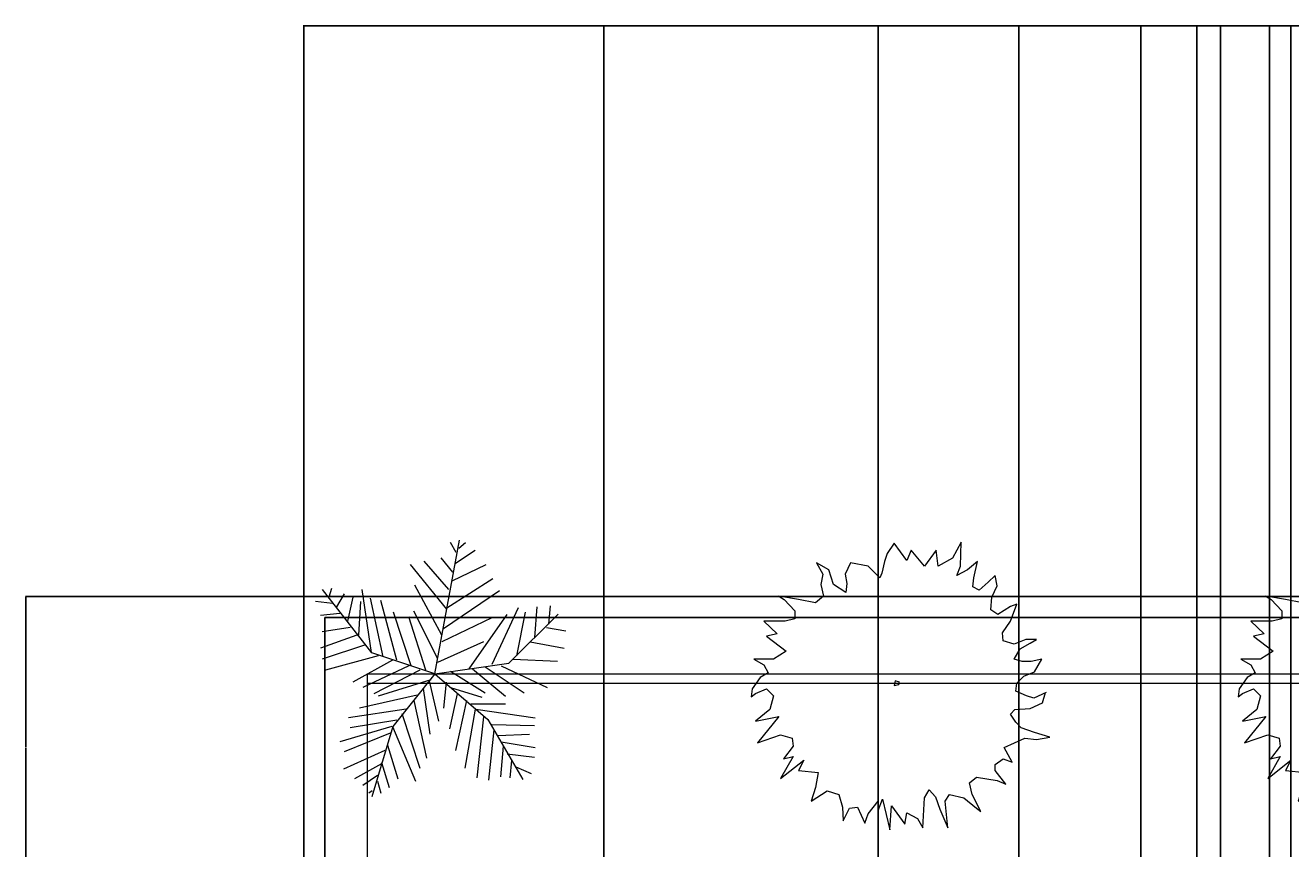
# Model space of a CAD drawing. Units: inches. Extents: x -4843 to -3402, y -164 to 3629.
# Tile 18 of 22: x -4843 to -4303, y 1042 to 1393. Entities that reach past the tile are written whole.
import ezdxf

# ---------------------------------------------------------------- set-up
doc = ezdxf.new("R2010")
doc.units = ezdxf.units.IN
for name, color, linetype, lineweight in [('A-ANNO-DIMS', 2, 'Continuous', 18), ('C-PROP', 7, 'Continuous', 25), ('L-PLNT-EDGE', 7, 'Continuous', 18), ('PLANTS', 3, 'Continuous', 13)]:
    doc.layers.add(name, color=color, linetype=linetype, lineweight=lineweight)
doc.styles.get("Standard").update_dxf_attribs({"font": 'arial.ttf'})
doc.dimstyles.get("Standard").update_dxf_attribs({"dimtxt": 0.18, "dimasz": 0.18, "dimexe": 0.18, "dimexo": 0.0625, "dimgap": 0.09, "dimtad": 0, "dimtih": 1, "dimtoh": 1, "dimdec": 4, "dimzin": 0, "dimdsep": 46, "dimtxsty": 'Standard', "dimcen": 0.09, "dimadec": 0, "dimazin": 0, "dimtfac": 1, "dimtdec": 4, "dimtofl": 0, "dimtmove": 0, "dimatfit": 3, "dimfxl": 1, "dimtolj": 1, "dimtzin": 0, "dimarcsym": 0})

# ---------------------------------------------------------------- blocks, each defined once
blk = doc.blocks.new('*U33')
for p, q in [((-258.7244, 1362.456), (-332.3336, 1421.4348)), ((0, 0), (-266.7, 1447.8)), ((-231.1146, 1315.2628), (-166.7002, 1421.4348)), ((-221.9198, 1197.3052), (-433.5526, 1338.8594)), ((-194.31, 1102.9442), (-65.4812, 1256.284)), ((-185.1152, 1008.5578), (-553.1612, 1185.4942)), ((-148.3106, 914.1968), (118.5418, 1220.9018)), ((-129.8956, 701.8528), (265.7602, 1185.4942)), ((-129.8956, 713.6638), (-626.7704, 1032.1544)), ((-74.7014, 418.7444), (219.7608, 961.39)), ((-93.091, 489.5342), (-700.3796, 902.3858)), ((685.8, 228.6), (1219.2, 914.4)), ((689.0258, 230.0224), (790.2448, 914.1968)), ((891.4384, 831.6214), (946.658, 572.1096)), ((983.4626, 867.0036), (1066.2666, 725.4494)), ((1121.4862, 925.9824), (1149.0706, 831.6214)), ((-1234.059, 536.7274), (-1252.4486, 737.2604)), ((-1105.2302, 725.4494), (-1077.6458, 395.1732)), ((-902.8176, 713.6638), (-617.5756, 100.2538)), ((412.9786, 147.447), (587.8068, 796.2392)), ((560.197, 182.8292), (698.2206, 819.8358)), ((808.6344, 784.4282), (827.0494, 418.7444)), ((1112.2914, 760.8316), (1296.3144, 784.4282)), ((-800.1, 114.3), (-1333.5, 647.7)), ((-976.4268, 666.4706), (-884.4026, 194.6402)), ((-369.1382, 53.086), (-783.1836, 642.874)), ((-617.5756, 607.4918), (-74.7014, 347.98)), ((-28.6766, 171.0436), (228.9556, 678.2816)), ((100.1268, 41.275), (284.1498, 619.2774)), ((256.5654, 88.4682), (449.7832, 666.4706)), ((1029.462, 654.685), (1241.0948, 631.0884)), ((-1206.4492, 501.3198), (-1418.082, 465.9376)), ((845.439, 418.7444), (1241.0948, 277.1902)), ((919.0482, 501.3198), (1222.6798, 454.152)), ((-1031.621, 347.98), (-1399.667, 277.1902)), ((-525.5514, 347.98), (-28.6766, 123.8504)), ((753.4148, 312.5978), (1222.6798, 159.2326)), ((-847.598, 159.2326), (-1326.0578, 135.636)), ((0, 0), (685.8, 228.6)), ((458.978, 147.447), (891.4384, -88.4682)), ((615.4166, 194.6402), (1185.8752, 41.275)), ((-718.7946, 88.4682), (-1215.644, -147.447)), ((-543.9664, 76.6572), (-967.2066, -206.4512)), ((0, 0), (-800.1, 114.3)), ((-405.9428, 53.086), (-764.794, -241.8334)), ((0, 0), (-571.5, -495.3)), ((-166.7002, 29.4894), (-543.9664, -206.4512)), ((0, 0), (457.2, -571.5)), ((164.5412, 41.275), (661.416, -218.2368)), ((284.1498, 88.4682), (781.0246, -147.447)), ((-120.7008, -88.4682), (-93.091, -371.5766)), ((63.3222, -76.6826), (-37.8714, -513.1308)), ((44.9326, -64.897), (615.4166, -241.8334)), ((-166.7002, -147.447), (-507.1618, -253.619)), ((-240.3094, -218.2368), (-157.5054, -595.7062)), ((127.7366, -159.258), (54.1274, -654.685)), ((192.151, -230.0224), (817.8292, -371.5766)), ((-442.7474, -383.3876), (-1086.8406, -477.7486)), ((-387.5278, -324.4088), (-764.794, -324.4088)), ((-433.5526, -383.3876), (-323.1134, -1020.3688)), ((-341.5284, -289.0012), (-221.9198, -831.6214)), ((228.9556, -289.0012), (90.932, -914.1968)), ((311.7596, -383.3876), (937.4378, -477.7486)), ((-571.5, -495.3), (-952.5, -1143)), ((-525.5514, -465.963), (-451.9422, -1126.5408)), ((357.759, -430.5554), (164.5412, -1020.3688)), ((412.9786, -501.3452), (919.0482, -583.9206)), ((-617.5756, -548.5384), (-1077.6458, -560.324)), ((-681.9646, -666.496), (-1022.4262, -654.685)), ((-635.9652, -607.5172), (-580.771, -1150.1374)), ((458.978, -572.1096), (210.5406, -1161.923)), ((457.2, -571.5), (685.8, -1333.5)), ((468.1982, -572.1096), (1029.462, -737.2604)), ((486.5878, -642.8994), (983.4626, -843.4324)), ((-718.7946, -737.2604), (-1086.8406, -796.2392)), ((-737.1842, -784.4536), (-709.5744, -1114.7298)), ((514.1976, -772.6426), (403.7838, -1138.3264)), ((-783.1836, -867.029), (-1077.6458, -902.4112)), ((-829.2084, -937.7934), (-810.7934, -1126.5408)), ((541.8074, -831.6214), (992.6574, -1032.1544)), ((-875.2078, -1008.5832), (-1040.8412, -1079.3476)), ((578.612, -961.39), (495.7826, -1232.7128)), ((578.612, -973.1756), (873.0488, -1138.3264)), ((624.6114, -1161.923), (587.8068, -1291.6916)), ((624.6114, -1102.9442), (781.0246, -1209.1162)), ((679.8056, -1268.095), (716.6102, -1291.6916))]:
    blk.add_line(p, q)
blk = doc.blocks.new('*U34')
for points in [[(0, 1540.256), (-77.4954, 1428.4452), (-106.5784, 1341.501), (-135.636, 1217.295), (-155.0162, 1167.6126), (-280.9748, 1291.8186), (-474.7514, 1329.0804), (-532.892, 1204.8744), (-513.5118, 1105.5096), (-523.1892, 1006.1194), (-658.8506, 1093.089), (-707.2884, 1254.5568), (-842.9244, 1329.0804), (-775.1064, 1204.8744), (-794.4866, 1093.089), (-765.429, 968.8576), (-852.6272, 894.334), (-1036.701, 931.5958), (-1249.8832, 968.8576), (-1191.7426, 931.5958), (-1075.4614, 807.3898), (-1075.4614, 720.4456), (-1182.0398, 695.6044), (-1414.5768, 695.6044), (-1269.238, 558.9524), (-1385.5192, 534.1112), (-1172.3624, 372.6434), (-1307.9984, 285.6992), (-1521.1552, 285.6992), (-1414.5768, 223.5962), (-1366.139, 136.652), (-1453.3372, 86.9442), (-1540.5354, -37.2618), (-1550.2382, -124.206), (-1501.775, -86.9442), (-1385.5192, -37.2618), (-1307.9984, -111.7854), (-1346.7588, -260.8326), (-1501.775, -385.064), (-1249.8832, -335.3816), (-1482.3948, -621.0554), (-1230.503, -534.1112), (-1104.5444, -571.373), (-1094.8416, -658.3172), (-1201.42, -794.9692), (-1094.8416, -770.128), (-1230.503, -1006.1194), (-978.5858, -807.3898), (-1036.701, -919.1752), (-823.5442, -944.0164), (-852.6272, -1105.4842), (-901.065, -1254.5568), (-726.6686, -1142.746), (-600.71, -1180.0078), (-561.9496, -1316.6598), (-552.2722, -1465.707), (-484.4542, -1329.0804), (-397.2306, -1316.6598), (-319.7352, -1490.5482), (-280.9748, -1391.1834), (-174.3964, -1254.5568), (-174.3964, -1353.9216), (-125.9586, -1229.7156), (-48.4378, -1565.0718), (-29.0576, -1304.2392), (116.2812, -1502.9688), (135.6614, -1378.7628), (251.9172, -1440.8658), (310.0578, -1540.2306), (329.438, -1217.295), (377.8758, -1130.3254), (445.6938, -1204.8744), (494.157, -1341.501), (581.3552, -1540.2306), (552.2722, -1254.5568), (600.71, -1180.0078), (755.7516, -1217.295), (891.3876, -1329.0804), (939.8254, -1366.3422), (842.9498, -1180.0078), (813.8668, -1055.8018), (891.3876, -993.6988), (1114.2472, -1030.9606), (1211.1228, -1068.2224), (1094.867, -919.1752), (1094.867, -857.0722), (1182.0652, -794.9692), (1278.9408, -832.231), (1191.7426, -670.7378), (1414.6022, -571.373), (1540.5608, -583.7936), (1685.8996, -558.9524), (1521.1806, -509.27), (1375.8418, -459.5876), (1317.7012, -397.4846), (1259.5606, -310.515), (1308.0238, -260.8326), (1472.7174, -248.412), (1608.3788, -186.309), (1637.4364, -74.5236)], [(1647.1392, -74.5236), (1511.4778, -136.6266), (1433.9824, -111.7854), (1317.7012, -62.103), (1327.404, 24.8412), (1404.8994, 99.3648), (1521.1806, 149.0726), (1598.676, 285.6992), (1482.4202, 260.858), (1385.5192, 260.858), (1298.321, 285.6992), (1366.139, 397.4846), (1472.7174, 459.5876), (1540.5608, 496.8494), (1424.2796, 496.8494), (1298.321, 447.167), (1182.0652, 484.4288), (1172.3624, 571.3984), (1259.5606, 695.6044), (1327.404, 881.9134), (1259.5606, 857.0722), (1123.9246, 770.128), (1046.4038, 819.8104), (1056.1066, 956.437), (1114.2472, 1080.6684), (1094.867, 1192.4538), (1017.3462, 1117.9302), (920.4452, 1030.9606), (852.6272, 1068.2478), (862.33, 1167.6126), (901.0904, 1341.501), (794.512, 1254.5568), (678.2308, 1192.4538), (716.9912, 1291.8186), (726.6686, 1552.6766), (629.793, 1378.7628), (474.7768, 1291.8186), (455.3966, 1465.7324), (329.438, 1291.8186), (184.0992, 1465.7324), (135.6614, 1353.9216), (0, 1540.256)]]:
    blk.add_lwpolyline(points)
blk.add_lwpolyline([(9.7028, 49.6824), (0, 0), (48.4378, 12.4206), (58.1406, 37.2618)], close=True)
blk = doc.blocks.new('*D60')
at = {"layer": 'A-ANNO-DIMS', "color": 0, "lineweight": -2, "transparency": 16777216}
for p, q in [((-4723.78, 1149.42), (-4723.78, 1392.95)), ((-4723.6, 1392.77), (-4333.07, 1392.77)), ((-3941.96, 1392.77), (-4332.5, 1392.77)), ((-3941.78, 1149.42), (-3941.78, 1392.95))]:
    blk.add_line(p, q, dxfattribs=at)
at = {"layer": 'A-ANNO-DIMS', "color": 0, "transparency": 16777216}
for points in [[(-4723.6, 1392.8), (-4723.6, 1392.74), (-4723.78, 1392.77)], [(-3941.96, 1392.8), (-3941.96, 1392.74), (-3941.78, 1392.77)]]:
    blk.add_solid(points, dxfattribs=at)
at = {"layer": 'Defpoints', "color": 0, "transparency": 16777216}
for p in [(-3941.78, 1392.77), (-4723.78, 1149.35), (-3941.78, 1149.35)]:
    blk.add_point(p, dxfattribs=at)
at = {"layer": 'A-ANNO-DIMS', "color": 0, "transparency": 16777216, "insert": (-4332.78, 1392.77), "char_height": 0.18, "attachment_point": 5}
blk.add_mtext('\\A1;782', dxfattribs=at)
blk = doc.blocks.new('*D68')
at = {"layer": 'A-ANNO-DIMS', "color": 0, "lineweight": -2, "transparency": 16777216}
for p, q in [((-4723.85, 1149.35), (-4842.55, 1149.35)), ((-4842.37, 1149.17), (-4842.37, 1085.04)), ((-4842.37, 1020.53), (-4842.37, 1084.67)), ((-4595.85, 1020.35), (-4842.55, 1020.35))]:
    blk.add_line(p, q, dxfattribs=at)
at = {"layer": 'A-ANNO-DIMS', "color": 0, "transparency": 16777216}
for points in [[(-4842.4, 1149.17), (-4842.34, 1149.17), (-4842.37, 1149.35)], [(-4842.4, 1020.53), (-4842.34, 1020.53), (-4842.37, 1020.35)]]:
    blk.add_solid(points, dxfattribs=at)
at = {"layer": 'Defpoints', "color": 0, "transparency": 16777216}
for p in [(-4723.78, 1149.35), (-4842.37, 1020.35), (-4595.78, 1020.35)]:
    blk.add_point(p, dxfattribs=at)
at = {"layer": 'A-ANNO-DIMS', "color": 0, "transparency": 16777216, "insert": (-4842.37, 1084.85), "char_height": 0.18, "attachment_point": 5}
blk.add_mtext('\\A1;129', dxfattribs=at)
blk = doc.blocks.new('*D69')
at = {"layer": 'A-ANNO-DIMS', "color": 0, "lineweight": -2, "transparency": 16777216}
for p, q in [((-4595.78, 1020.42), (-4595.78, 1392.95)), ((-4595.6, 1392.77), (-4537.56, 1392.77)), ((-4478.96, 1392.77), (-4537, 1392.77)), ((-4478.78, 1020.42), (-4478.78, 1392.95))]:
    blk.add_line(p, q, dxfattribs=at)
at = {"layer": 'A-ANNO-DIMS', "color": 0, "transparency": 16777216}
for points in [[(-4595.6, 1392.8), (-4595.6, 1392.74), (-4595.78, 1392.77)], [(-4478.96, 1392.8), (-4478.96, 1392.74), (-4478.78, 1392.77)]]:
    blk.add_solid(points, dxfattribs=at)
at = {"layer": 'Defpoints', "color": 0, "transparency": 16777216}
for p in [(-4478.78, 1392.77), (-4595.78, 1020.35), (-4478.78, 1020.35)]:
    blk.add_point(p, dxfattribs=at)
at = {"layer": 'A-ANNO-DIMS', "color": 0, "transparency": 16777216, "insert": (-4537.28, 1392.77), "char_height": 0.18, "attachment_point": 5}
blk.add_mtext('\\A1;117', dxfattribs=at)
blk = doc.blocks.new('*D70')
at = {"layer": 'A-ANNO-DIMS', "color": 0, "lineweight": -2, "transparency": 16777216}
for p, q in [((-4418.78, 1020.42), (-4418.78, 1392.95)), ((-4418.6, 1392.77), (-4393, 1392.77)), ((-4366.96, 1392.77), (-4392.56, 1392.77)), ((-4366.78, 1020.42), (-4366.78, 1392.95))]:
    blk.add_line(p, q, dxfattribs=at)
at = {"layer": 'A-ANNO-DIMS', "color": 0, "transparency": 16777216}
for points in [[(-4418.6, 1392.8), (-4418.6, 1392.74), (-4418.78, 1392.77)], [(-4366.96, 1392.8), (-4366.96, 1392.74), (-4366.78, 1392.77)]]:
    blk.add_solid(points, dxfattribs=at)
at = {"layer": 'Defpoints', "color": 0, "transparency": 16777216}
for p in [(-4366.78, 1392.77), (-4418.78, 1020.35), (-4366.78, 1020.35)]:
    blk.add_point(p, dxfattribs=at)
at = {"layer": 'A-ANNO-DIMS', "color": 0, "transparency": 16777216, "insert": (-4392.78, 1392.77), "char_height": 0.18, "attachment_point": 5}
blk.add_mtext('\\A1;52', dxfattribs=at)
blk = doc.blocks.new('*D71')
at = {"layer": 'A-ANNO-DIMS', "color": 0, "lineweight": -2, "transparency": 16777216}
for p, q in [((-4342.78, 1020.42), (-4342.78, 1392.95)), ((-4342.6, 1392.77), (-4327.48, 1392.77)), ((-4311.96, 1392.77), (-4327.08, 1392.77)), ((-4311.78, 1011.42), (-4311.78, 1392.95))]:
    blk.add_line(p, q, dxfattribs=at)
at = {"layer": 'A-ANNO-DIMS', "color": 0, "transparency": 16777216}
for points in [[(-4342.6, 1392.8), (-4342.6, 1392.74), (-4342.78, 1392.77)], [(-4311.96, 1392.8), (-4311.96, 1392.74), (-4311.78, 1392.77)]]:
    blk.add_solid(points, dxfattribs=at)
at = {"layer": 'Defpoints', "color": 0, "transparency": 16777216}
for p in [(-4311.78, 1392.77), (-4342.78, 1020.35), (-4311.78, 1011.35)]:
    blk.add_point(p, dxfattribs=at)
at = {"layer": 'A-ANNO-DIMS', "color": 0, "transparency": 16777216, "insert": (-4327.28, 1392.77), "char_height": 0.18, "attachment_point": 5}
blk.add_mtext('\\A1;31', dxfattribs=at)
blk = doc.blocks.new('*D72')
at = {"layer": 'A-ANNO-DIMS', "color": 0, "lineweight": -2, "transparency": 16777216}
for p, q in [((-4302.78, 1011.42), (-4302.78, 1392.95)), ((-4302.6, 1392.77), (-4285, 1392.77)), ((-4266.96, 1392.77), (-4284.56, 1392.77)), ((-4266.78, 1020.42), (-4266.78, 1392.95))]:
    blk.add_line(p, q, dxfattribs=at)
at = {"layer": 'A-ANNO-DIMS', "color": 0, "transparency": 16777216}
for points in [[(-4302.6, 1392.8), (-4302.6, 1392.74), (-4302.78, 1392.77)], [(-4266.96, 1392.8), (-4266.96, 1392.74), (-4266.78, 1392.77)]]:
    blk.add_solid(points, dxfattribs=at)
at = {"layer": 'Defpoints', "color": 0, "transparency": 16777216}
for p in [(-4266.78, 1392.77), (-4266.78, 1020.35), (-4302.78, 1011.35)]:
    blk.add_point(p, dxfattribs=at)
at = {"layer": 'A-ANNO-DIMS', "color": 0, "transparency": 16777216, "insert": (-4284.78, 1392.77), "char_height": 0.18, "attachment_point": 5}
blk.add_mtext('\\A1;36', dxfattribs=at)
blk = doc.blocks.new('*D81')
at = {"layer": 'A-ANNO-DIMS', "color": 0, "lineweight": -2, "transparency": 16777216}
for p, q in [((-4332.78, 86.42), (-4332.78, 1392.95)), ((-4332.6, 1392.77), (-4168.61, 1392.77)), ((-4003.86, 1392.77), (-4167.86, 1392.77)), ((-4003.68, 86.42), (-4003.68, 1392.95))]:
    blk.add_line(p, q, dxfattribs=at)
at = {"layer": 'A-ANNO-DIMS', "color": 0, "transparency": 16777216}
for points in [[(-4332.6, 1392.8), (-4332.6, 1392.74), (-4332.78, 1392.77)], [(-4003.86, 1392.8), (-4003.86, 1392.74), (-4003.68, 1392.77)]]:
    blk.add_solid(points, dxfattribs=at)
at = {"layer": 'Defpoints', "color": 0, "transparency": 16777216}
for p in [(-4003.68, 1392.77), (-4332.78, 86.35), (-4003.68, 86.35)]:
    blk.add_point(p, dxfattribs=at)
at = {"layer": 'A-ANNO-DIMS', "color": 0, "transparency": 16777216, "insert": (-4168.23, 1392.77), "char_height": 0.18, "attachment_point": 5}
blk.add_mtext('\\A1;329.1', dxfattribs=at)

msp = doc.modelspace()

# ---------------------------------------------------------------- linework, layer by layer
at = {"layer": 'C-PROP'}
for p, q in [((-4723.78, 1149.35), (-4723.78, 86.35)), ((-4723.78, 1149.35), (-3941.78, 1149.35)), ((-4714.78, 1140.35), (-4714.78, 95.35)), ((-4714.78, 1140.35), (-3950.78, 1140.35))]:
    msp.add_line(p, q, dxfattribs=at)
at = {"layer": 'L-PLNT-EDGE'}
for p, q in [((-4696.78, 1116.35), (-3974.78, 1116.35)), ((-4696.78, 1116.35), (-4696.78, 95.35)), ((-4696.78, 1112.35), (-3978.78, 1112.35))]:
    msp.add_line(p, q, dxfattribs=at)

# ---------------------------------------------------------------- block references
at = {"layer": 'PLANTS', "xscale": -0.0393700787401575, "yscale": 0.0393700787401575, "zscale": 0.0393700787401575, "rotation": 359.9999999999706}
msp.add_blockref('*U33', (-4667.81, 1116.35), dxfattribs=at)
at = {"layer": 'PLANTS', "xscale": 0.0393700787401575, "yscale": 0.0393700787401575, "zscale": 0.0393700787401575}
for p in [(-4471.91, 1111.38), (-4264.15, 1111.38)]:
    msp.add_blockref('*U34', p, dxfattribs=at)

# ---------------------------------------------------------------- dimensions: what is measured, and where the dimension line sits
at = {"layer": 'A-ANNO-DIMS'}
for base, p1, p2, override, picture, middle in [((-3941.78, 1392.77), (-4723.78, 1149.35), (-3941.78, 1149.35), {"dimdec": 0, "dimlfac": 1, "dimrnd": 0, "dimzin": 0, "dimdsep": 46, "dimlunit": 2}, '*D60', (-4332.78, 1392.77)), ((-4478.78, 1392.77), (-4595.78, 1020.35), (-4478.78, 1020.35), {"dimdec": 0, "dimlfac": 1, "dimrnd": 0, "dimzin": 0, "dimdsep": 46, "dimlunit": 2}, '*D69', (-4537.28, 1392.77)), ((-4366.78, 1392.77), (-4418.78, 1020.35), (-4366.78, 1020.35), {"dimdec": 0, "dimlfac": 1, "dimrnd": 0, "dimzin": 0, "dimdsep": 46, "dimlunit": 2}, '*D70', (-4392.78, 1392.77)), ((-4311.78, 1392.77), (-4342.78, 1020.35), (-4311.78, 1011.35), {"dimdec": 0, "dimlfac": 1, "dimrnd": 0, "dimzin": 0, "dimdsep": 46, "dimlunit": 2}, '*D71', (-4327.28, 1392.77)), ((-4003.68, 1392.77), (-4332.78, 86.35), (-4003.68, 86.35), {"dimdec": 1, "dimlfac": 1, "dimrnd": 0, "dimzin": 0, "dimdsep": 46, "dimlunit": 2}, '*D81', (-4168.23, 1392.77)), ((-4266.78, 1392.77), (-4302.78, 1011.35), (-4266.78, 1020.35), {"dimdec": 0, "dimlfac": 1, "dimrnd": 0, "dimzin": 0, "dimdsep": 46, "dimlunit": 2}, '*D72', (-4284.78, 1392.77))]:
    dim = msp.add_linear_dim(base=base, p1=p1, p2=p2, dimstyle='Standard', override=override, dxfattribs=at)
    dim.commit()
    dim.dimension.update_dxf_attribs({"geometry": picture, "text_midpoint": middle})
dim = msp.add_linear_dim(base=(-4842.37, 1020.35), p1=(-4723.78, 1149.35), p2=(-4595.78, 1020.35), angle=90, dimstyle='Standard', override={"dimdec": 0, "dimlfac": 1, "dimrnd": 0, "dimzin": 0, "dimdsep": 46, "dimlunit": 2}, dxfattribs=at)
dim.commit()
dim.dimension.update_dxf_attribs({"geometry": '*D68', "text_midpoint": (-4842.37, 1084.85)})

doc.saveas('drawing.dxf')
